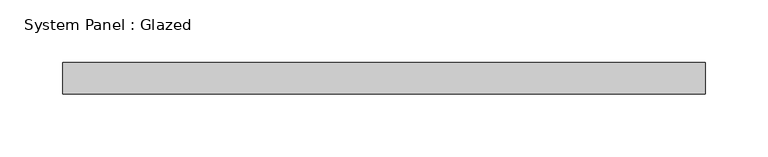
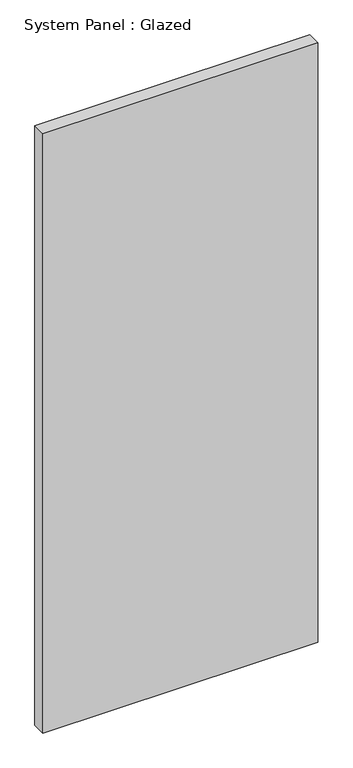
"""IFC4 building model written with IfcOpenShell, lengths in millimetres: plate geometry, System Panel : Glazed."""

from ifc_helpers import new_model, si_unit, origin, origin_with_axes, place, context, project, spatial, polyline, outline, extrude, source, transform, mapped, element, save


def system_panel_glazed_4a8c201a(model_context):
    return source(origin(), model_context, "Body", "SweptSolid", [
        extrude(outline(polyline([(257.175, 19.05), (-257.175, 19.05), (-257.175, 44.45), (257.175, 44.45), (257.175, 19.05)])), origin_with_axes(), (0.0, 0.0, 1.0), 1185.0463864),
    ])


if __name__ == "__main__":
    model = new_model("IFC4")
    model_context = context("Model", 3, world=origin())
    ifc_project = project(units=[si_unit("LENGTHUNIT", "METRE", prefix="MILLI")], contexts=[model_context])
    site = spatial("IfcSite", under=ifc_project)
    building = spatial("IfcBuilding", under=site)
    placement = place(None, origin())
    system_panel_glazed_shape = system_panel_glazed_4a8c201a(model_context)
    element("IfcPlate", 1, ObjectType="System Panel : Glazed", at=placement, inside=building, context=model_context, shape_type="MappedRepresentation", body=[
        mapped(system_panel_glazed_shape, transform((0.0, 0.0, 0.0), x_axis=(1.0, 0.0, 0.0), y_axis=(0.0, 1.0, 0.0), z_axis=(0.0, 0.0, 1.0))),
    ])
    save(model, "model.ifc")

# Revit data of these elements
# Type "System Panel : Glazed"
#   Construction Type Id = "GSP4R"
#   Analytic Construction = "1/8 in Pilkington single glazing"
#   Visual Light Transmittance = 0.9
#   Solar Heat Gain Coefficient = 0.86
#   Heat Transfer Coefficient (U) = 1.18115 BTU/(h·ft²·°F)
#   Define Thermal Properties by = 1
# Element 1 (IfcPlate, "System Panel : Glazed")
#   Materials on its faces: "Glass"
# Materials
#   "Glass": class "Glass", colour RGB 0 128 192, transparency 0.75, Description = "Soda Lime Glass", Cost = 0
